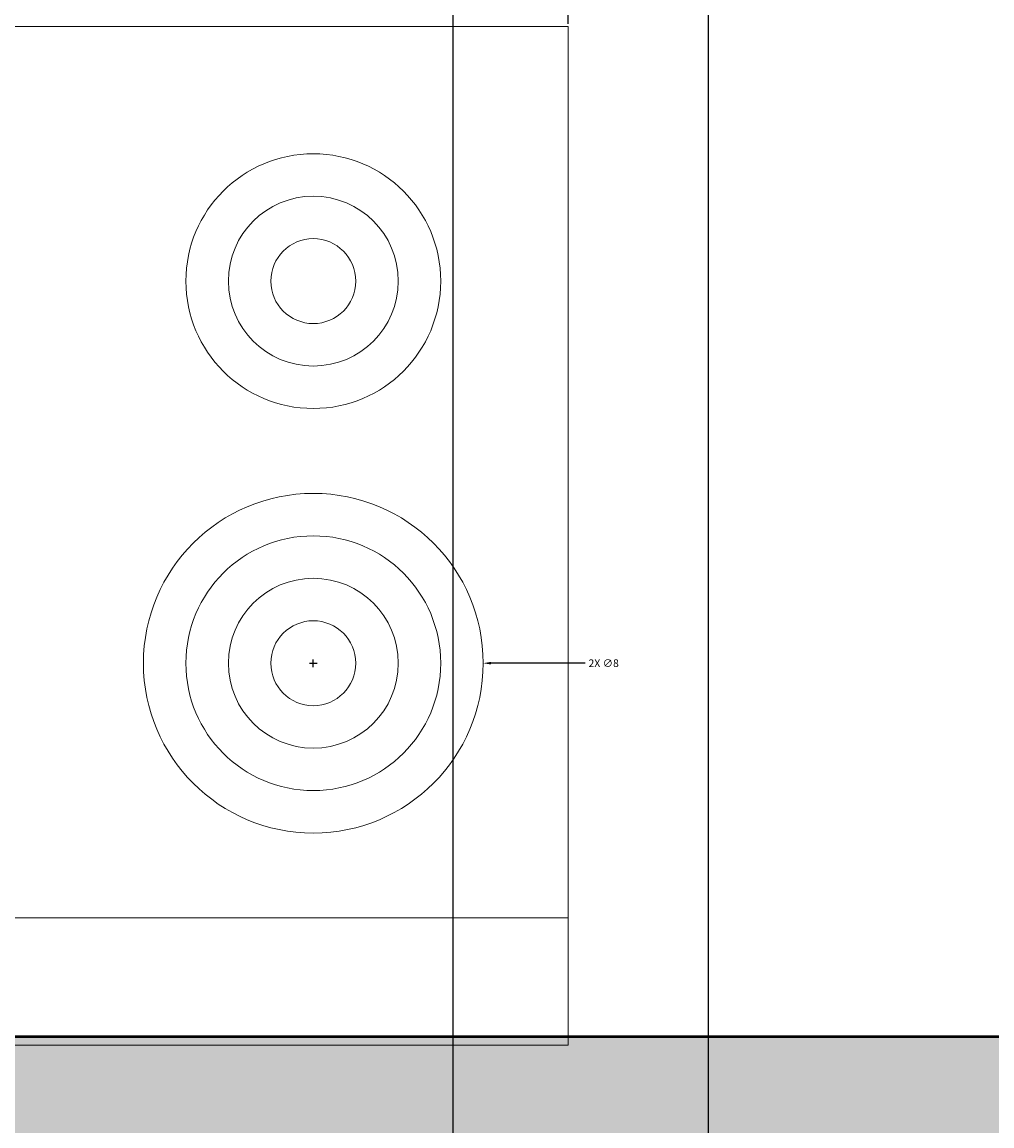
# Model space of a CAD drawing. Units: inches. Extents: x 2307 to 2544, y 2171 to 2540.
# Tile 31 of 52: x 2476 to 2498, y 2317 to 2343. Entities that reach past the tile are written whole.
import ezdxf

# ---------------------------------------------------------------- set-up
doc = ezdxf.new("R2010")
doc.units = ezdxf.units.IN
for name, color, linetype, lineweight in [('A-ANNO-DIMS', 2, 'Continuous', 18), ('A-EQPM', 8, 'Continuous', 18), ('A-WALL', 7, 'Continuous', 50)]:
    doc.layers.add(name, color=color, linetype=linetype, lineweight=lineweight)
doc.layers.add('A-WALL-PATT', color=18, linetype='Continuous', lineweight=13, true_color=0x000000)
doc.styles.get("Standard").update_dxf_attribs({"font": 'arial.ttf'})
doc.dimstyles.get("Standard").update_dxf_attribs({"dimtxt": 0.18, "dimasz": 0.18, "dimexe": 0.18, "dimexo": 0.0625, "dimgap": 0.09, "dimtad": 0, "dimtih": 1, "dimtoh": 1, "dimdec": 4, "dimzin": 0, "dimdsep": 46, "dimtxsty": 'Standard', "dimcen": 0.09, "dimadec": 0, "dimazin": 0, "dimtfac": 1, "dimtdec": 4, "dimtofl": 0, "dimtmove": 0, "dimatfit": 3, "dimfxl": 1, "dimtolj": 1, "dimtzin": 0, "dimarcsym": 0})

# ---------------------------------------------------------------- blocks, each defined once
blk = doc.blocks.new('Range-Oven - 30 in top')
blk.add_line((0, -3), (30, -3))
blk.add_lwpolyline([(0, -24), (0, 0), (30, 0), (30, -24)], close=True)
for centre, radius in [((6, -9), 4), ((6, -9), 3), ((24, -9), 3), ((6, -9), 2), ((24, -9), 2), ((6, -9), 1), ((24, -9), 1), ((24, -18), 4), ((6, -18), 3), ((24, -18), 3), ((6, -18), 2), ((24, -18), 2), ((6, -18), 1), ((24, -18), 1)]:
    blk.add_circle(centre, radius)
blk = doc.blocks.new('*D30')
at = {"layer": 'A-ANNO-DIMS', "color": 0, "lineweight": -2, "transparency": 16777216}
for p, q in [((2458.401, 2343.369), (2458.401, 2347.987)), ((2458.581, 2347.807), (2472.705, 2347.807)), ((2488.221, 2347.807), (2474.097, 2347.807)), ((2488.401, 2343.369), (2488.401, 2347.987))]:
    blk.add_line(p, q, dxfattribs=at)
at = {"layer": 'A-ANNO-DIMS', "color": 0, "transparency": 16777216}
for points in [[(2458.581, 2347.837), (2458.581, 2347.777), (2458.401, 2347.807)], [(2488.221, 2347.837), (2488.221, 2347.777), (2488.401, 2347.807)]]:
    blk.add_solid(points, dxfattribs=at)
at = {"layer": 'Defpoints', "color": 0, "transparency": 16777216}
for p in [(2458.401, 2347.807), (2458.401, 2343.307), (2488.401, 2343.307)]:
    blk.add_point(p, dxfattribs=at)
at = {"layer": 'A-ANNO-DIMS', "color": 0, "transparency": 16777216, "insert": (2473.401, 2347.807), "char_height": 0.18, "attachment_point": 5}
blk.add_mtext('\\A1;RANGE 30', dxfattribs=at)
blk = doc.blocks.new('*D54')
at = {"layer": 'A-ANNO-DIMS', "color": 0, "lineweight": -2, "transparency": 16777216}
for p, q in [((2461.696, 2435.447), (2461.696, 2171.18)), ((2491.696, 2435.447), (2491.696, 2171.18)), ((2461.876, 2171.36), (2476.477, 2171.36)), ((2491.516, 2171.36), (2476.914, 2171.36))]:
    blk.add_line(p, q, dxfattribs=at)
at = {"layer": 'A-ANNO-DIMS', "color": 0, "transparency": 16777216}
for points in [[(2461.876, 2171.39), (2461.876, 2171.33), (2461.696, 2171.36)], [(2491.516, 2171.39), (2491.516, 2171.33), (2491.696, 2171.36)]]:
    blk.add_solid(points, dxfattribs=at)
at = {"layer": 'Defpoints', "color": 0, "transparency": 16777216}
for p in [(2461.696, 2435.51), (2491.696, 2435.51), (2491.696, 2171.36)]:
    blk.add_point(p, dxfattribs=at)
at = {"layer": 'A-ANNO-DIMS', "color": 0, "transparency": 16777216, "insert": (2476.696, 2171.36), "char_height": 0.18, "attachment_point": 5}
blk.add_mtext('\\A1;30', dxfattribs=at)
blk = doc.blocks.new('*D59')
at = {"layer": 'A-ANNO-DIMS', "color": 0, "lineweight": -2, "transparency": 16777216}
for p, q in [((2455.696, 2315.572), (2455.696, 2540.345)), ((2485.696, 2315.572), (2485.696, 2540.345)), ((2455.876, 2540.165), (2470.477, 2540.165)), ((2485.516, 2540.165), (2470.914, 2540.165))]:
    blk.add_line(p, q, dxfattribs=at)
at = {"layer": 'A-ANNO-DIMS', "color": 0, "transparency": 16777216}
for points in [[(2455.876, 2540.195), (2455.876, 2540.135), (2455.696, 2540.165)], [(2485.516, 2540.195), (2485.516, 2540.135), (2485.696, 2540.165)]]:
    blk.add_solid(points, dxfattribs=at)
at = {"layer": 'Defpoints', "color": 0, "transparency": 16777216}
for p in [(2455.696, 2540.165), (2455.696, 2315.51), (2485.696, 2315.51)]:
    blk.add_point(p, dxfattribs=at)
at = {"layer": 'A-ANNO-DIMS', "color": 0, "transparency": 16777216, "insert": (2470.696, 2540.165), "char_height": 0.18, "attachment_point": 5}
blk.add_mtext('\\A1;30', dxfattribs=at)
blk = doc.blocks.new('*D70')
at = {"layer": 'A-ANNO-DIMS', "color": 0, "lineweight": -2, "transparency": 16777216}
for p, q in [((2482.311, 2328.307), (2482.491, 2328.307)), ((2482.401, 2328.217), (2482.401, 2328.397)), ((2488.801, 2328.307), (2486.581, 2328.307))]:
    blk.add_line(p, q, dxfattribs=at)
at = {"layer": 'A-ANNO-DIMS', "color": 0, "transparency": 16777216}
blk.add_solid([(2486.581, 2328.337), (2486.581, 2328.277), (2486.401, 2328.307)], dxfattribs=at)
at = {"layer": 'Defpoints', "color": 0, "transparency": 16777216}
for p in [(2478.401, 2328.307), (2486.401, 2328.307)]:
    blk.add_point(p, dxfattribs=at)
at = {"layer": 'A-ANNO-DIMS', "color": 0, "transparency": 16777216, "insert": (2489.238, 2328.307), "char_height": 0.18, "attachment_point": 5}
blk.add_mtext('\\A1;2X ∅8', dxfattribs=at)

msp = doc.modelspace()

# ---------------------------------------------------------------- hatches: boundary and pattern name
at = {"layer": 'A-WALL-PATT'}
h = msp.add_hatch(color=256, dxfattribs=at)
h.dxf.hatch_style = 1
h.paths.add_polyline_path([(2433.6935, 2199.5096), (2415.6423, 2199.5096), (2415.6423, 2190.5096), (2433.7832, 2190.5096)], flags=17)
h.paths.add_polyline_path([(2367.6423, 2199.5096), (2335.6958, 2199.5096), (2335.6958, 2307.3983), (2326.6958, 2307.3983), (2326.6958, 2190.5096), (2367.6423, 2190.5096)])
h.paths.add_polyline_path([(2524.6958, 2520.5096), (2496.7832, 2520.5096), (2496.7832, 2515.5149), (2472.7832, 2515.5149), (2472.7832, 2520.5096), (2415.4028, 2520.5096), (2415.4028, 2511.5096), (2451.6958, 2511.5096), (2451.6958, 2439.5096), (2451.6958, 2391.5096), (2445.6958, 2391.5096), (2445.6958, 2387.5096), (2455.6958, 2387.5096), (2455.6958, 2435.5096), (2461.6958, 2435.5096), (2461.6958, 2439.5096), (2455.6958, 2439.5096), (2455.6958, 2511.5096), (2515.6958, 2511.5096), (2515.6958, 2439.5096), (2491.6958, 2439.5096), (2491.6958, 2435.5096), (2515.6958, 2435.5096), (2515.6958, 2319.5096), (2451.6958, 2319.5096), (2451.6958, 2281.5096), (2481.6958, 2281.5096), (2481.6958, 2225.5096), (2485.6958, 2225.5096), (2485.6958, 2285.5096), (2455.6958, 2285.5096), (2455.6958, 2315.5096), (2515.6958, 2315.5096), (2515.6958, 2199.5096), (2469.6952, 2199.5096), (2469.785, 2190.5096), (2524.6958, 2190.5096)])

# ---------------------------------------------------------------- linework, layer by layer
at = {"layer": 'A-WALL'}
msp.add_line((2515.6958, 2319.5096), (2451.6958, 2319.5096), dxfattribs=at)

# ---------------------------------------------------------------- block references
at = {"layer": 'A-EQPM', "rotation": 180}
msp.add_blockref('Range-Oven - 30 in top', (2488.4011, 2319.3068), dxfattribs=at)

# ---------------------------------------------------------------- dimensions: what is measured, and where the dimension line sits
at = {"layer": 'A-ANNO-DIMS'}
for base, p1, p2, picture, middle in [((2455.6958, 2540.1649), (2485.6958, 2315.5096), (2455.6958, 2315.5096), '*D59', (2470.6958, 2540.1649)), ((2491.6958, 2171.3596), (2461.6958, 2435.5096), (2491.6958, 2435.5096), '*D54', (2476.6958, 2171.3596))]:
    dim = msp.add_linear_dim(base=base, p1=p1, p2=p2, dimstyle='Standard', override={"dimdec": 0, "dimlfac": 1, "dimrnd": 0, "dimzin": 0, "dimdsep": 46, "dimlunit": 2}, dxfattribs=at)
    dim.commit()
    dim.dimension.update_dxf_attribs({"geometry": picture, "text_midpoint": middle})
dim = msp.add_linear_dim(base=(2458.4011, 2347.8068), p1=(2488.4011, 2343.3068), p2=(2458.4011, 2343.3068), angle=180, text='RANGE <>', dimstyle='Standard', override={"dimdec": 0, "dimlfac": 1, "dimrnd": 0, "dimzin": 0, "dimdsep": 46, "dimlunit": 2}, dxfattribs=at)
dim.commit()
dim.dimension.update_dxf_attribs({"geometry": '*D30', "text_midpoint": (2473.4011, 2347.8068)})
dim = msp.add_diameter_dim_2p(p1=(2478.4011, 2328.3066), p2=(2486.4011, 2328.307), text='2X <>', dimstyle='Standard', override={"dimdec": 0, "dimlfac": 1, "dimrnd": 0, "dimzin": 0, "dimdsep": 46, "dimlunit": 2}, dxfattribs=at)
dim.commit()
dim.dimension.update_dxf_attribs({"geometry": '*D70', "text_midpoint": (2488.8011, 2328.3071), "dimtype": 163})

doc.saveas('drawing.dxf')
